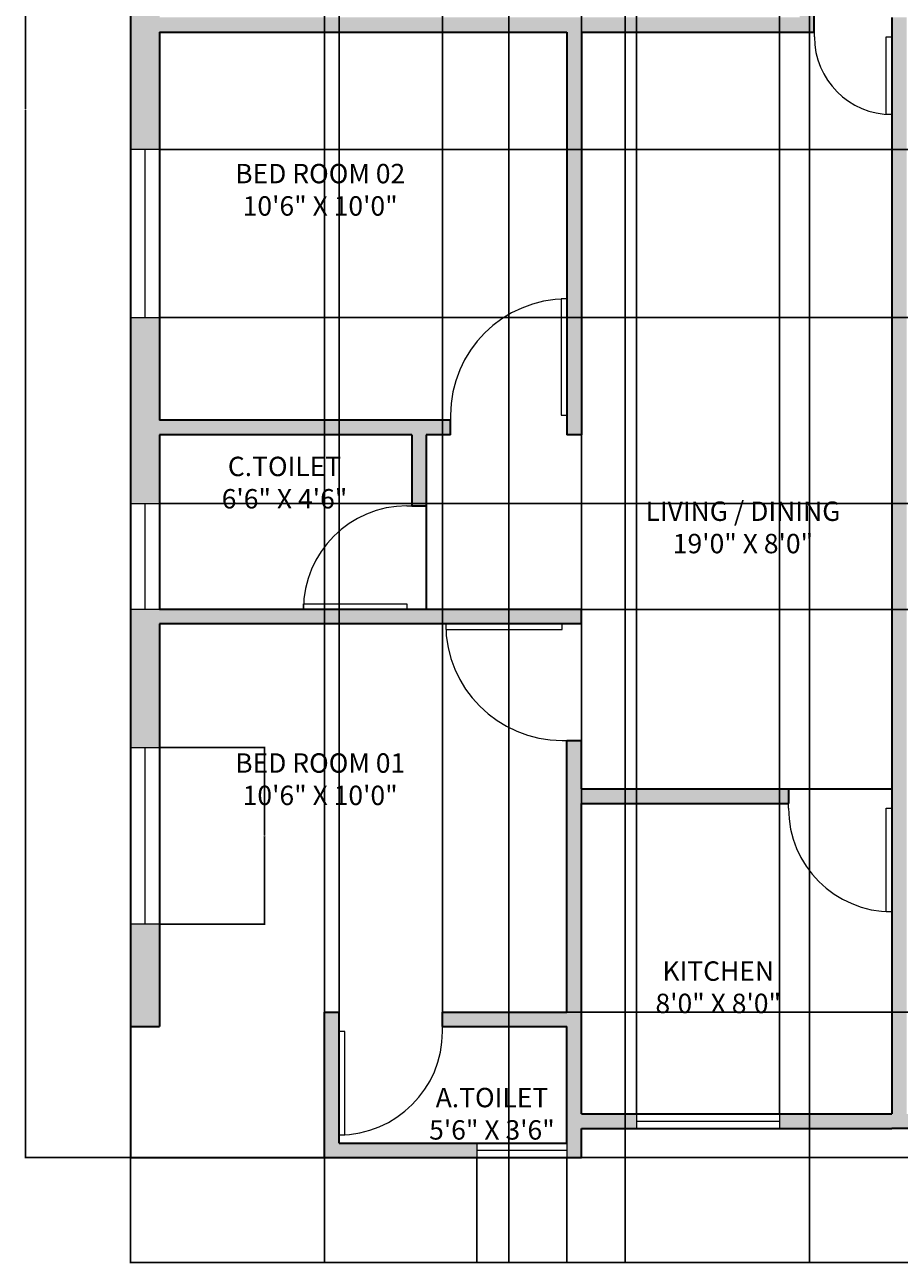
# Model space of a CAD drawing. Units: inches. Extents: x 2510 to 3056, y 673 to 1386.
# Tile 1 of 4: x 2511 to 2781, y 673 to 1056. Entities that reach past the tile are written whole.
import ezdxf

# ---------------------------------------------------------------- set-up
doc = ezdxf.new("R2010")
doc.units = ezdxf.units.IN
for name, color, linetype, lineweight in [('A-ANNO-DIMS', 2, 'Continuous', 18), ('A-AREA-IDEN', 7, 'Continuous', 18), ('A-DOOR', 3, 'Continuous', 18), ('A-GLAZ', 4, 'Continuous', 18), ('A-WALL', 7, 'Continuous', 35), ('A-WALL-PATT', 252, 'Continuous', 13)]:
    doc.layers.add(name, color=color, linetype=linetype, lineweight=lineweight)
doc.styles.get("Standard").update_dxf_attribs({"font": 'arial.ttf'})
doc.dimstyles.get("Standard").update_dxf_attribs({"dimtxt": 0.18, "dimasz": 0.18, "dimexe": 0.18, "dimexo": 0.0625, "dimgap": 0.09, "dimtad": 0, "dimtih": 1, "dimtoh": 1, "dimdec": 4, "dimzin": 0, "dimdsep": 46, "dimtxsty": 'Standard', "dimcen": 0.09, "dimadec": 0, "dimazin": 0, "dimtfac": 1, "dimtdec": 4, "dimtofl": 0, "dimtmove": 0, "dimatfit": 3, "dimfxl": 1, "dimtolj": 1, "dimtzin": 0, "dimarcsym": 0})

# ---------------------------------------------------------------- blocks, each defined once
blk = doc.blocks.new('*U8')
for p, q in [((-24, 0), (-24, 6)), ((0, 0), (0, 6))]:
    blk.add_line(p, q)
blk.add_lwpolyline([(0, 0), (0, -24), (-1.75, -24), (-1.75, 0)], close=True)
blk.add_arc((0, 0), 24, 180, 270)
blk = doc.blocks.new('*U4')
for p, q in [((0, 0), (0, -6)), ((-36, 0), (-36, -6))]:
    blk.add_line(p, q)
blk.add_lwpolyline([(0, 0), (0, 36), (-1.75, 36), (-1.75, 0)], close=True)
blk.add_arc((0, 0), 36, 90, 180)
blk = doc.blocks.new('*U9')
for p, q in [((-32, 0), (-32, 6)), ((0, 0), (0, 6))]:
    blk.add_line(p, q)
blk.add_lwpolyline([(0, 0), (0, -32), (-1.75, -32), (-1.75, 0)], close=True)
blk.add_arc((0, 0), 32, 180, 270)
blk = doc.blocks.new('*U2')
for p, q in [((0, 0), (0, -6)), ((32, 0), (32, -6))]:
    blk.add_line(p, q)
blk.add_lwpolyline([(0, 0), (0, 32), (1.75, 32), (1.75, 0)], close=True)
blk.add_arc((0, 0), 32, 0, 90)
blk = doc.blocks.new('*U5')
for p, q in [((0, 0), (0, 6)), ((32, 0), (32, 6))]:
    blk.add_line(p, q)
blk.add_lwpolyline([(0, 0), (0, -32), (1.75, -32), (1.75, 0)], close=True)
blk.add_arc((0, 0), 32, 270, 0)
blk = doc.blocks.new('*D12')
at = {"layer": 'A-ANNO-DIMS', "color": 0, "lineweight": -2, "transparency": 16777216}
for p, q in [((2543.13, 1353.59), (2510.53, 1353.59)), ((2510.71, 1353.41), (2510.71, 1029.77)), ((2510.71, 705.77), (2510.71, 1029.4)), ((2543.13, 705.59), (2510.53, 705.59))]:
    blk.add_line(p, q, dxfattribs=at)
at = {"layer": 'A-ANNO-DIMS', "color": 0, "transparency": 16777216}
for points in [[(2510.68, 1353.41), (2510.74, 1353.41), (2510.71, 1353.59)], [(2510.68, 705.77), (2510.74, 705.77), (2510.71, 705.59)]]:
    blk.add_solid(points, dxfattribs=at)
at = {"layer": 'Defpoints', "color": 0, "transparency": 16777216}
for p in [(2510.71, 1353.59), (2543.19, 1353.59), (2543.19, 705.59)]:
    blk.add_point(p, dxfattribs=at)
at = {"layer": 'A-ANNO-DIMS', "color": 0, "transparency": 16777216, "insert": (2510.71, 1029.59), "char_height": 0.18, "attachment_point": 5}
blk.add_mtext('\\A1;648', dxfattribs=at)
blk = doc.blocks.new('*D13')
at = {"layer": 'A-ANNO-DIMS', "color": 0, "lineweight": -2, "transparency": 16777216}
for p, q in [((2543.19, 705.52), (2543.19, 672.93)), ((3023.19, 705.52), (3023.19, 672.93)), ((2543.37, 673.11), (2782.9, 673.11)), ((3023.01, 673.11), (2783.48, 673.11))]:
    blk.add_line(p, q, dxfattribs=at)
at = {"layer": 'A-ANNO-DIMS', "color": 0, "transparency": 16777216}
for points in [[(2543.37, 673.14), (2543.37, 673.08), (2543.19, 673.11)], [(3023.01, 673.14), (3023.01, 673.08), (3023.19, 673.11)]]:
    blk.add_solid(points, dxfattribs=at)
at = {"layer": 'Defpoints', "color": 0, "transparency": 16777216}
for p in [(2543.19, 705.59), (3023.19, 705.59), (3023.19, 673.11)]:
    blk.add_point(p, dxfattribs=at)
at = {"layer": 'A-ANNO-DIMS', "color": 0, "transparency": 16777216, "insert": (2783.19, 673.11), "char_height": 0.18, "attachment_point": 5}
blk.add_mtext('\\A1;480', dxfattribs=at)
blk = doc.blocks.new('*D33')
at = {"layer": 'A-ANNO-DIMS', "color": 0, "lineweight": -2, "transparency": 16777216}
for p, q in [((2552.25, 832.37), (2584.85, 832.37)), ((2584.67, 832.19), (2584.67, 805.22)), ((2584.67, 777.9), (2584.67, 804.86)), ((2552.25, 777.72), (2584.85, 777.72))]:
    blk.add_line(p, q, dxfattribs=at)
at = {"layer": 'A-ANNO-DIMS', "color": 0, "transparency": 16777216}
for points in [[(2584.64, 832.19), (2584.7, 832.19), (2584.67, 832.37)], [(2584.64, 777.9), (2584.7, 777.9), (2584.67, 777.72)]]:
    blk.add_solid(points, dxfattribs=at)
at = {"layer": 'Defpoints', "color": 0, "transparency": 16777216}
for p in [(2552.19, 832.37), (2552.19, 777.72), (2584.67, 777.72)]:
    blk.add_point(p, dxfattribs=at)
at = {"layer": 'A-ANNO-DIMS', "color": 0, "transparency": 16777216, "insert": (2584.67, 805.04), "char_height": 0.18, "attachment_point": 5}
blk.add_mtext('\\A1;54.65', dxfattribs=at)
blk = doc.blocks.new('*D34')
at = {"layer": 'A-ANNO-DIMS', "color": 0, "lineweight": -2, "transparency": 16777216}
for p, q in [((2552.25, 907.81), (3055.85, 907.81)), ((3055.67, 907.63), (3055.67, 891.63)), ((3055.67, 875.27), (3055.67, 891.27)), ((2552.25, 875.09), (3055.85, 875.09))]:
    blk.add_line(p, q, dxfattribs=at)
at = {"layer": 'A-ANNO-DIMS', "color": 0, "transparency": 16777216}
for points in [[(3055.64, 907.63), (3055.7, 907.63), (3055.67, 907.81)], [(3055.64, 875.27), (3055.7, 875.27), (3055.67, 875.09)]]:
    blk.add_solid(points, dxfattribs=at)
at = {"layer": 'Defpoints', "color": 0, "transparency": 16777216}
for p in [(2552.19, 907.81), (3055.67, 907.81), (2552.19, 875.09)]:
    blk.add_point(p, dxfattribs=at)
at = {"layer": 'A-ANNO-DIMS', "color": 0, "transparency": 16777216, "insert": (3055.67, 891.45), "char_height": 0.18, "attachment_point": 5}
blk.add_mtext('\\A1;32.72', dxfattribs=at)
blk = doc.blocks.new('*D35')
at = {"layer": 'A-ANNO-DIMS', "color": 0, "lineweight": -2, "transparency": 16777216}
for p, q in [((2552.25, 1017.32), (3055.85, 1017.32)), ((3055.67, 1017.14), (3055.67, 991.52)), ((3055.67, 965.53), (3055.67, 991.15)), ((2552.25, 965.35), (3055.85, 965.35))]:
    blk.add_line(p, q, dxfattribs=at)
at = {"layer": 'A-ANNO-DIMS', "color": 0, "transparency": 16777216}
for points in [[(3055.64, 1017.14), (3055.7, 1017.14), (3055.67, 1017.32)], [(3055.64, 965.53), (3055.7, 965.53), (3055.67, 965.35)]]:
    blk.add_solid(points, dxfattribs=at)
at = {"layer": 'Defpoints', "color": 0, "transparency": 16777216}
for p in [(2552.19, 1017.32), (3055.67, 1017.32), (2552.19, 965.35)]:
    blk.add_point(p, dxfattribs=at)
at = {"layer": 'A-ANNO-DIMS', "color": 0, "transparency": 16777216, "insert": (3055.67, 991.34), "char_height": 0.18, "attachment_point": 5}
blk.add_mtext('\\A1;51.97', dxfattribs=at)
blk = doc.blocks.new('*D40')
at = {"layer": 'A-ANNO-DIMS', "color": 0, "lineweight": -2, "transparency": 16777216}
for p, q in [((2682.69, 719.15), (2682.69, 1386.25)), ((2699.74, 719.15), (2699.74, 1386.25)), ((2682.87, 1386.07), (2690.76, 1386.07)), ((2699.56, 1386.07), (2691.67, 1386.07))]:
    blk.add_line(p, q, dxfattribs=at)
at = {"layer": 'A-ANNO-DIMS', "color": 0, "transparency": 16777216}
for points in [[(2682.87, 1386.1), (2682.87, 1386.04), (2682.69, 1386.07)], [(2699.56, 1386.1), (2699.56, 1386.04), (2699.74, 1386.07)]]:
    blk.add_solid(points, dxfattribs=at)
at = {"layer": 'Defpoints', "color": 0, "transparency": 16777216}
for p in [(2699.74, 1386.07), (2682.69, 719.09), (2699.74, 719.09)]:
    blk.add_point(p, dxfattribs=at)
at = {"layer": 'A-ANNO-DIMS', "color": 0, "transparency": 16777216, "insert": (2691.22, 1386.07), "char_height": 0.18, "attachment_point": 5}
blk.add_mtext('\\A1;17.045', dxfattribs=at)
blk = doc.blocks.new('*D41')
at = {"layer": 'A-ANNO-DIMS', "color": 0, "lineweight": -2, "transparency": 16777216}
for p, q in [((2699.74, 719.15), (2699.74, 1386.25)), ((2743.88, 719.15), (2743.88, 1386.25)), ((2699.92, 1386.07), (2721.41, 1386.07)), ((2743.7, 1386.07), (2722.21, 1386.07))]:
    blk.add_line(p, q, dxfattribs=at)
at = {"layer": 'A-ANNO-DIMS', "color": 0, "transparency": 16777216}
for points in [[(2699.92, 1386.1), (2699.92, 1386.04), (2699.74, 1386.07)], [(2743.7, 1386.1), (2743.7, 1386.04), (2743.88, 1386.07)]]:
    blk.add_solid(points, dxfattribs=at)
at = {"layer": 'Defpoints', "color": 0, "transparency": 16777216}
for p in [(2743.88, 1386.07), (2699.74, 719.09), (2743.88, 719.09)]:
    blk.add_point(p, dxfattribs=at)
at = {"layer": 'A-ANNO-DIMS', "color": 0, "transparency": 16777216, "insert": (2721.81, 1386.07), "char_height": 0.18, "attachment_point": 5}
blk.add_mtext('\\A1;44.14', dxfattribs=at)
blk = doc.blocks.new('*D45')
at = {"layer": 'A-ANNO-DIMS', "color": 0, "lineweight": -2, "transparency": 16777216}
for p, q in [((2660.19, 1208.02), (2660.19, 672.93)), ((2696.19, 1208.02), (2696.19, 672.93)), ((2660.37, 673.11), (2677.97, 673.11)), ((2696.01, 673.11), (2678.41, 673.11))]:
    blk.add_line(p, q, dxfattribs=at)
at = {"layer": 'A-ANNO-DIMS', "color": 0, "transparency": 16777216}
for points in [[(2660.37, 673.14), (2660.37, 673.08), (2660.19, 673.11)], [(2696.01, 673.14), (2696.01, 673.08), (2696.19, 673.11)]]:
    blk.add_solid(points, dxfattribs=at)
at = {"layer": 'Defpoints', "color": 0, "transparency": 16777216}
for p in [(2660.19, 1208.09), (2696.19, 1208.09), (2696.19, 673.11)]:
    blk.add_point(p, dxfattribs=at)
at = {"layer": 'A-ANNO-DIMS', "color": 0, "transparency": 16777216, "insert": (2678.19, 673.11), "char_height": 0.18, "attachment_point": 5}
blk.add_mtext('\\A1;36', dxfattribs=at)
blk = doc.blocks.new('*D46')
at = {"layer": 'A-ANNO-DIMS', "color": 0, "lineweight": -2, "transparency": 16777216}
for p, q in [((2753.19, 1256.02), (2753.19, 672.93)), ((2785.19, 1256.02), (2785.19, 672.93)), ((2753.37, 673.11), (2768.97, 673.11)), ((2785.01, 673.11), (2769.41, 673.11))]:
    blk.add_line(p, q, dxfattribs=at)
at = {"layer": 'A-ANNO-DIMS', "color": 0, "transparency": 16777216}
for points in [[(2753.37, 673.14), (2753.37, 673.08), (2753.19, 673.11)], [(2785.01, 673.14), (2785.01, 673.08), (2785.19, 673.11)]]:
    blk.add_solid(points, dxfattribs=at)
at = {"layer": 'Defpoints', "color": 0, "transparency": 16777216}
for p in [(2753.19, 1256.09), (2785.19, 1256.09), (2785.19, 673.11)]:
    blk.add_point(p, dxfattribs=at)
at = {"layer": 'A-ANNO-DIMS', "color": 0, "transparency": 16777216, "insert": (2769.19, 673.11), "char_height": 0.18, "attachment_point": 5}
blk.add_mtext('\\A1;32', dxfattribs=at)
blk = doc.blocks.new('*D50')
at = {"layer": 'A-ANNO-DIMS', "color": 0, "lineweight": -2, "transparency": 16777216}
for p, q in [((2607.69, 750.65), (2607.69, 1386.25)), ((2639.69, 750.65), (2639.69, 1386.25)), ((2607.87, 1386.07), (2623.47, 1386.07)), ((2639.51, 1386.07), (2623.91, 1386.07))]:
    blk.add_line(p, q, dxfattribs=at)
at = {"layer": 'A-ANNO-DIMS', "color": 0, "transparency": 16777216}
for points in [[(2607.87, 1386.1), (2607.87, 1386.04), (2607.69, 1386.07)], [(2639.51, 1386.1), (2639.51, 1386.04), (2639.69, 1386.07)]]:
    blk.add_solid(points, dxfattribs=at)
at = {"layer": 'Defpoints', "color": 0, "transparency": 16777216}
for p in [(2639.69, 1386.07), (2607.69, 750.59), (2639.69, 750.59)]:
    blk.add_point(p, dxfattribs=at)
at = {"layer": 'A-ANNO-DIMS', "color": 0, "transparency": 16777216, "insert": (2623.69, 1386.07), "char_height": 0.18, "attachment_point": 5}
blk.add_mtext('\\A1;32', dxfattribs=at)
blk = doc.blocks.new('*D51')
at = {"layer": 'A-ANNO-DIMS', "color": 0, "lineweight": -2, "transparency": 16777216}
for p, q in [((2650.28, 705.52), (2650.28, 672.93)), ((2678.19, 705.52), (2678.19, 672.93)), ((2650.46, 673.11), (2663.77, 673.11)), ((2678.01, 673.11), (2664.7, 673.11))]:
    blk.add_line(p, q, dxfattribs=at)
at = {"layer": 'A-ANNO-DIMS', "color": 0, "transparency": 16777216}
for points in [[(2650.46, 673.14), (2650.46, 673.08), (2650.28, 673.11)], [(2678.01, 673.14), (2678.01, 673.08), (2678.19, 673.11)]]:
    blk.add_solid(points, dxfattribs=at)
at = {"layer": 'Defpoints', "color": 0, "transparency": 16777216}
for p in [(2650.28, 705.59), (2678.19, 705.59), (2678.19, 673.11)]:
    blk.add_point(p, dxfattribs=at)
at = {"layer": 'A-ANNO-DIMS', "color": 0, "transparency": 16777216, "insert": (2664.23, 673.11), "char_height": 0.18, "attachment_point": 5}
blk.add_mtext('\\A1;27.916', dxfattribs=at)
blk = doc.blocks.new('*D52')
at = {"layer": 'A-ANNO-DIMS', "color": 0, "lineweight": -2, "transparency": 16777216}
for p, q in [((2603.19, 705.52), (2603.19, 672.93)), ((2650.28, 705.52), (2650.28, 672.93)), ((2603.37, 673.11), (2626.34, 673.11)), ((2650.1, 673.11), (2627.13, 673.11))]:
    blk.add_line(p, q, dxfattribs=at)
at = {"layer": 'A-ANNO-DIMS', "color": 0, "transparency": 16777216}
for points in [[(2603.37, 673.14), (2603.37, 673.08), (2603.19, 673.11)], [(2650.1, 673.14), (2650.1, 673.08), (2650.28, 673.11)]]:
    blk.add_solid(points, dxfattribs=at)
at = {"layer": 'Defpoints', "color": 0, "transparency": 16777216}
for p in [(2603.19, 705.59), (2650.28, 705.59), (2650.28, 673.11)]:
    blk.add_point(p, dxfattribs=at)
at = {"layer": 'A-ANNO-DIMS', "color": 0, "transparency": 16777216, "insert": (2626.73, 673.11), "char_height": 0.18, "attachment_point": 5}
blk.add_mtext('\\A1;47.08', dxfattribs=at)
blk = doc.blocks.new('*D53')
at = {"layer": 'A-ANNO-DIMS', "color": 0, "lineweight": -2, "transparency": 16777216}
for p, q in [((2682.75, 714.59), (3055.85, 714.59)), ((3055.67, 714.41), (3055.67, 710.27)), ((3055.67, 705.77), (3055.67, 709.9)), ((2682.75, 705.59), (3055.85, 705.59))]:
    blk.add_line(p, q, dxfattribs=at)
at = {"layer": 'A-ANNO-DIMS', "color": 0, "transparency": 16777216}
for points in [[(3055.64, 714.41), (3055.7, 714.41), (3055.67, 714.59)], [(3055.64, 705.77), (3055.7, 705.77), (3055.67, 705.59)]]:
    blk.add_solid(points, dxfattribs=at)
at = {"layer": 'Defpoints', "color": 0, "transparency": 16777216}
for p in [(2682.69, 714.59), (3055.67, 714.59), (2682.69, 705.59)]:
    blk.add_point(p, dxfattribs=at)
at = {"layer": 'A-ANNO-DIMS', "color": 0, "transparency": 16777216, "insert": (3055.67, 710.09), "char_height": 0.18, "attachment_point": 5}
blk.add_mtext('\\A1;9', dxfattribs=at)
blk = doc.blocks.new('*D54')
at = {"layer": 'A-ANNO-DIMS', "color": 0, "lineweight": -2, "transparency": 16777216}
for p, q in [((2678.25, 750.59), (3055.85, 750.59)), ((3055.67, 750.41), (3055.67, 732.77)), ((3055.67, 714.77), (3055.67, 732.4)), ((2682.75, 714.59), (3055.85, 714.59))]:
    blk.add_line(p, q, dxfattribs=at)
at = {"layer": 'A-ANNO-DIMS', "color": 0, "transparency": 16777216}
for points in [[(3055.64, 750.41), (3055.7, 750.41), (3055.67, 750.59)], [(3055.64, 714.77), (3055.7, 714.77), (3055.67, 714.59)]]:
    blk.add_solid(points, dxfattribs=at)
at = {"layer": 'Defpoints', "color": 0, "transparency": 16777216}
for p in [(2678.19, 750.59), (3055.67, 750.59), (2682.69, 714.59)]:
    blk.add_point(p, dxfattribs=at)
at = {"layer": 'A-ANNO-DIMS', "color": 0, "transparency": 16777216, "insert": (3055.67, 732.59), "char_height": 0.18, "attachment_point": 5}
blk.add_mtext('\\A1;36', dxfattribs=at)
blk = doc.blocks.new('*D57')
at = {"layer": 'A-ANNO-DIMS', "color": 0, "lineweight": -2, "transparency": 16777216}
for p, q in [((2543.19, 705.65), (2543.19, 1386.25)), ((2603.19, 705.65), (2603.19, 1386.25)), ((2543.37, 1386.07), (2572.97, 1386.07)), ((2603.01, 1386.07), (2573.41, 1386.07))]:
    blk.add_line(p, q, dxfattribs=at)
at = {"layer": 'A-ANNO-DIMS', "color": 0, "transparency": 16777216}
for points in [[(2543.37, 1386.1), (2543.37, 1386.04), (2543.19, 1386.07)], [(2603.01, 1386.1), (2603.01, 1386.04), (2603.19, 1386.07)]]:
    blk.add_solid(points, dxfattribs=at)
at = {"layer": 'Defpoints', "color": 0, "transparency": 16777216}
for p in [(2603.19, 1386.07), (2543.19, 705.59), (2603.19, 705.59)]:
    blk.add_point(p, dxfattribs=at)
at = {"layer": 'A-ANNO-DIMS', "color": 0, "transparency": 16777216, "insert": (2573.19, 1386.07), "char_height": 0.18, "attachment_point": 5}
blk.add_mtext('\\A1;60', dxfattribs=at)

msp = doc.modelspace()

# ---------------------------------------------------------------- hatches: boundary and pattern name
at = {"layer": 'A-WALL-PATT'}
h = msp.add_hatch(color=256, dxfattribs=at)
h.dxf.hatch_style = 1
h.paths.add_polyline_path([(2580.5162, 1353.5862), (2543.1924, 1353.5862), (2543.1924, 1311.5591), (2552.1924, 1311.5591), (2552.1924, 1344.5862), (2580.5162, 1344.5862)])
h.paths.add_polyline_path([(2720.7125, 1353.5862), (2648.0497, 1353.5862), (2648.0497, 1344.5862), (2696.1924, 1344.5862), (2696.1924, 1208.0862), (2700.6924, 1208.0862), (2700.6924, 1256.0862), (2716.6924, 1256.0862), (2716.6924, 1260.5862), (2700.6924, 1260.5862), (2700.6924, 1344.5862), (2720.7125, 1344.5862)])
h.paths.add_polyline_path([(2762.4727, 1353.5862), (2748.6924, 1353.5862), (2748.6924, 1344.5862), (2748.6924, 1256.0862), (2753.1924, 1256.0862), (2753.1924, 1262.0862), (2753.1924, 1294.0862), (2753.1924, 1344.5862), (2762.4727, 1344.5862)])
h.paths.add_polyline_path([(2863.5016, 1353.5862), (2808.6621, 1353.5862), (2808.6621, 1344.5862), (2825.1924, 1344.5862), (2825.1924, 1260.5862), (2785.1924, 1260.5862), (2785.1924, 1256.0862), (2825.1924, 1256.0862), (2825.1924, 1248.5862), (2829.6924, 1248.5862), (2829.6924, 1344.5862), (2863.5016, 1344.5862)])
h.paths.add_polyline_path([(2966.1924, 1353.5862), (2915.7284, 1353.5862), (2915.7284, 1344.5862), (2961.6924, 1344.5862), (2961.6924, 1212.5862), (2897.6924, 1212.5862), (2897.6924, 1208.0862), (2961.6924, 1208.0862), (2961.6924, 1193.4346), (2966.1924, 1193.4346), (2966.1924, 1208.0862)])
h.paths.add_polyline_path([(2660.1924, 1212.5862), (2552.1924, 1212.5862), (2552.1924, 1254.8401), (2543.1924, 1254.8401), (2543.1924, 1168.7504), (2552.1924, 1168.7504), (2552.1924, 1208.0862), (2660.1924, 1208.0862)])
h.paths.add_polyline_path([(3023.1924, 1160.0862), (2966.1924, 1160.0862), (2966.1924, 1165.033), (2961.6924, 1165.033), (2961.6924, 1160.0862), (2865.6924, 1160.0862), (2865.6924, 1212.5862), (2825.1924, 1212.5862), (2825.1924, 1208.0862), (2861.1924, 1208.0862), (2861.1924, 1160.0862), (2750.1527, 1160.0862), (2750.1527, 1155.5862), (2754.6527, 1155.5862), (2966.1924, 1155.5862), (3014.1924, 1155.5862), (3014.1924, 1136.4806), (3023.1924, 1136.4806)])
h.paths.add_polyline_path([(3023.1924, 1090.8839), (3014.1924, 1090.8839), (3014.1924, 1058.0862), (2807.1924, 1058.0862), (2807.1924, 1053.5862), (2879.1924, 1053.5862), (2879.1924, 929.0862), (2883.6924, 929.0862), (2883.6924, 935.0862), (2883.6924, 971.0862), (2883.6924, 1053.5862), (3014.1924, 1053.5862), (3014.1924, 1028.0329), (3023.1924, 1028.0329)])
h.paths.add_polyline_path([(3023.1924, 970.6943), (3014.1924, 970.6943), (3014.1924, 933.5862), (2919.6924, 933.5862), (2919.6924, 929.0862), (2927.1924, 929.0862), (2927.1924, 907.0862), (2931.6924, 907.0862), (2931.6924, 929.0862), (3014.1924, 929.0862), (3014.1924, 918.5377), (3023.1924, 918.5377)])
h.paths.add_polyline_path([(3023.1924, 886.219), (3014.1924, 886.219), (3014.1924, 875.0862), (2927.1924, 875.0862), (2879.1924, 875.0862), (2879.1924, 870.5862), (2885.1924, 870.5862), (2921.1924, 870.5862), (3014.1924, 870.5862), (3014.1924, 835.4806), (3023.1924, 835.4806)])
h.paths.add_polyline_path([(3023.1924, 775.6299), (3014.1924, 775.6299), (3014.1924, 746.0862), (3023.1924, 746.0862)])
h.paths.add_polyline_path([(2958.6924, 750.5862), (2954.1924, 750.5862), (2954.1924, 744.5862), (2954.1924, 716.5862), (2954.1924, 710.0862), (2910.6841, 710.0862), (2910.6841, 705.5862), (2958.6924, 705.5862)])
h.paths.add_polyline_path([(2926.1924, 750.5862), (2883.6924, 750.5862), (2883.6924, 834.5862), (2879.1924, 834.5862), (2879.1924, 819.5862), (2815.1924, 819.5862), (2815.1924, 815.0862), (2879.1924, 815.0862), (2879.1924, 746.0862), (2879.1924, 719.0862), (2862.8388, 719.0862), (2862.8388, 714.5862), (2879.1924, 714.5862), (2879.1924, 705.5862), (2883.6924, 705.5862), (2883.6924, 710.0862), (2883.6924, 746.0862), (2926.1924, 746.1758)])
h.paths.add_polyline_path([(2682.6924, 815.0862), (2746.6924, 815.0862), (2746.6924, 819.5862), (2682.6924, 819.5862), (2682.6924, 834.5862), (2678.1924, 834.5862), (2678.1924, 750.5862), (2639.6924, 750.5862), (2639.6924, 746.0862), (2678.1924, 746.0862), (2678.1924, 710.0862), (2678.1924, 705.5862), (2682.6924, 705.5862), (2682.6924, 714.5862), (2699.7376, 714.5862), (2699.7376, 719.0862), (2682.6924, 719.0862), (2682.6924, 746.0862)])
h.paths.add_polyline_path([(2650.2761, 710.0862), (2607.6924, 710.0862), (2607.6924, 750.5862), (2603.1924, 750.5862), (2603.1924, 705.5862), (2607.6924, 705.5862), (2650.2761, 705.5862)])
h.paths.add_polyline_path([(2552.1924, 777.7158), (2543.1924, 777.7158), (2543.1924, 746.0862), (2552.1924, 746.0862)])
h.paths.add_polyline_path([(2828.3093, 719.0862), (2783.1924, 719.0862), (2783.1924, 815.0862), (2783.1924, 1058.0862), (2778.6924, 1058.0862), (2778.6924, 815.0862), (2778.6924, 719.0862), (2743.8813, 719.0862), (2743.8813, 714.5862), (2778.6924, 714.5862), (2828.3093, 714.5862)])
h.paths.add_polyline_path([(2642.1924, 933.5862), (2552.1924, 933.5862), (2552.1924, 965.3494), (2543.1924, 965.3494), (2543.1924, 907.809), (2552.1924, 907.809), (2552.1924, 929.0862), (2630.1924, 929.0862), (2630.1924, 907.0862), (2634.6924, 907.0862), (2634.6924, 929.0862), (2642.1924, 929.0862)])
h.paths.add_polyline_path([(2682.6924, 875.0862), (2552.1924, 875.0862), (2543.1924, 875.0862), (2543.1924, 832.3664), (2552.1924, 832.3664), (2552.1924, 870.5862), (2634.6924, 870.5862), (2682.6924, 870.5862)])
h.paths.add_polyline_path([(2754.6527, 1119.5862), (2750.1527, 1119.5862), (2750.1527, 1058.0862), (2552.1924, 1058.0862), (2552.1924, 1104.0128), (2543.1924, 1104.0128), (2543.1924, 1017.3235), (2552.1924, 1017.3235), (2552.1924, 1053.5862), (2678.1924, 1053.5862), (2678.1924, 929.0862), (2682.6924, 929.0862), (2682.6924, 1053.5862), (2754.6527, 1053.5862)])

# ---------------------------------------------------------------- linework, layer by layer
at = {"layer": 'A-GLAZ'}
for p, q in [((2543.1924, 1017.3235), (2552.1924, 1017.3235)), ((2547.6924, 965.3494), (2547.6924, 1017.3235)), ((2543.1924, 965.3494), (2552.1924, 965.3494)), ((2543.1924, 907.809), (2552.1924, 907.809)), ((2547.6924, 875.0862), (2547.6924, 907.809)), ((2552.1924, 875.0862), (2543.1924, 875.0862)), ((2543.1924, 832.3664), (2552.1924, 832.3664)), ((2547.6924, 777.7158), (2547.6924, 832.3664)), ((2552.1924, 777.7158), (2543.1924, 777.7158)), ((2699.7376, 719.0862), (2699.7376, 714.5862)), ((2699.7376, 716.8362), (2743.8813, 716.8362)), ((2743.8813, 719.0862), (2743.8813, 714.5862)), ((2650.2761, 710.0862), (2650.2761, 705.5862)), ((2678.1924, 710.0862), (2678.1924, 705.5862)), ((2650.2761, 707.8362), (2678.1924, 707.8362))]:
    msp.add_line(p, q, dxfattribs=at)
at = {"layer": 'A-WALL'}
for p, q in [((2543.1924, 1353.5862), (2543.1924, 705.5862)), ((2754.6527, 1053.5862), (2754.6527, 1119.5862)), ((2778.6924, 1058.0862), (2778.6924, 815.0862)), ((2552.1924, 1053.5862), (2678.1924, 1053.5862)), ((2552.1924, 1053.5862), (2552.1924, 933.5862)), ((2678.1924, 1053.5862), (2678.1924, 929.0862)), ((2682.6924, 1053.5862), (2682.6924, 929.0862)), ((2682.6924, 1053.5862), (2754.6527, 1053.5862)), ((2642.1924, 933.5862), (2552.1924, 933.5862)), ((2642.1924, 929.0862), (2642.1924, 933.5862)), ((2630.1924, 929.0862), (2552.1924, 929.0862)), ((2552.1924, 929.0862), (2552.1924, 875.0862)), ((2630.1924, 929.0862), (2630.1924, 907.0862)), ((2634.6924, 929.0862), (2634.6924, 875.0862)), ((2642.1924, 929.0862), (2634.6924, 929.0862)), ((2682.6924, 929.0862), (2678.1924, 929.0862)), ((2630.1924, 907.0862), (2634.6924, 907.0862)), ((2682.6924, 875.0862), (2552.1924, 875.0862)), ((2682.6924, 870.5862), (2682.6924, 875.0862)), ((2634.6924, 870.5862), (2552.1924, 870.5862)), ((2552.1924, 870.5862), (2552.1924, 746.0862)), ((2682.6924, 870.5862), (2634.6924, 870.5862)), ((2678.1924, 750.5862), (2678.1924, 834.5862)), ((2678.1924, 834.5862), (2682.6924, 834.5862)), ((2682.6924, 819.5862), (2682.6924, 834.5862)), ((2682.6924, 819.5862), (2778.6924, 819.5862)), ((2746.6924, 819.5862), (2746.6924, 815.0862)), ((2682.6924, 746.0862), (2682.6924, 815.0862)), ((2682.6924, 815.0862), (2746.6924, 815.0862)), ((2778.6924, 815.0862), (2778.6924, 719.0862)), ((2603.1924, 750.5862), (2607.6924, 750.5862)), ((2603.1924, 705.5862), (2603.1924, 750.5862)), ((2607.6924, 710.0862), (2607.6924, 750.5862)), ((2639.6924, 746.0862), (2639.6924, 750.5862)), ((2639.6924, 750.5862), (2678.1924, 750.5862)), ((2543.1924, 746.0862), (2552.1924, 746.0862)), ((2639.6924, 746.0862), (2678.1924, 746.0862)), ((2678.1924, 710.0862), (2678.1924, 746.0862)), ((2682.6924, 719.0862), (2682.6924, 746.0862)), ((2682.6924, 719.0862), (2778.6924, 719.0862)), ((2682.6924, 705.5862), (2682.6924, 714.5862)), ((2682.6924, 714.5862), (2778.6924, 714.5862)), ((2879.1924, 714.5862), (2778.6924, 714.5862)), ((2607.6924, 710.0862), (2678.1924, 710.0862)), ((2543.1924, 705.5862), (2603.1924, 705.5862)), ((2603.1924, 705.5862), (2607.6924, 705.5862)), ((2607.6924, 705.5862), (2678.1924, 705.5862)), ((2678.1924, 705.5862), (2682.6924, 705.5862))]:
    msp.add_line(p, q, dxfattribs=at)

# ---------------------------------------------------------------- block references
at = {"layer": 'A-DOOR'}
for name, p in [('*U8', (2778.6924, 1052.0862)), ('*U4', (2678.1924, 935.0862)), ('*U9', (2778.6924, 813.5862)), ('*U5', (2607.6924, 744.5862))]:
    msp.add_blockref(name, p, dxfattribs=at)
at = {"layer": 'A-DOOR', "rotation": 90}
for name, p in [('*U2', (2628.6924, 875.0862)), ('*U4', (2676.6924, 870.5862))]:
    msp.add_blockref(name, p, dxfattribs=at)

# ---------------------------------------------------------------- texts
at = {"layer": 'A-AREA-IDEN', "char_height": 6, "attachment_point": 1}
for s, width, insert in [('\\pxqc;BED ROOM 02\\P10\'6" X 10\'0"', 59.569763, (2572.0833, 1012.8204)), ('\\pxqc;C.TOILET\\P6\'6" X 4\'6"', 59.569763, (2561.0461, 922.2835)), ('\\pxqc;LIVING / DINING\\P19\'0" X 8\'0"', 75.716205, (2694.7584, 908.4349)), ('\\pxqc;BED ROOM 01\\P10\'6" X 10\'0"', 59.569763, (2572.0833, 830.5806)), ('\\pxqc;KITCHEN\\P\\pt7;8\'0" X 8\'0"', 59.569763, (2695.1869, 766.2581)), ('\\pxqc;A.TOILET\\P5\'6" X 3\'6"', 40.931341, (2634.522, 727.1456))]:
    msp.add_mtext_dynamic_manual_height_columns(s, width=width, gutter_width=12.5, heights=[0], dxfattribs=dict(at, insert=insert))

# ---------------------------------------------------------------- dimensions: what is measured, and where the dimension line sits
at = {"layer": 'A-ANNO-DIMS'}
for base, p1, p2, override, picture, middle in [((2603.1924, 1386.0667), (2543.1924, 705.5862), (2603.1924, 705.5862), {"dimdec": 0, "dimlfac": 1, "dimrnd": 0, "dimzin": 0, "dimdsep": 46, "dimlunit": 2}, '*D57', (2573.1924, 1386.0667)), ((2639.6924, 1386.0667), (2607.6924, 750.5862), (2639.6924, 750.5862), {"dimdec": 0, "dimlfac": 1, "dimrnd": 0, "dimzin": 0, "dimdsep": 46, "dimlunit": 2}, '*D50', (2623.6924, 1386.0667)), ((2699.7376, 1386.0667), (2682.6924, 719.0862), (2699.7376, 719.0862), {"dimdec": 3, "dimlfac": 1, "dimrnd": 0, "dimzin": 0, "dimdsep": 46, "dimlunit": 2}, '*D40', (2691.215, 1386.0667)), ((2743.8813, 1386.0667), (2699.7376, 719.0862), (2743.8813, 719.0862), {"dimdec": 2, "dimlfac": 1, "dimrnd": 0, "dimzin": 0, "dimdsep": 46, "dimlunit": 2}, '*D41', (2721.8095, 1386.0667)), ((2785.1924, 673.1057), (2753.1924, 1256.0862), (2785.1924, 1256.0862), {"dimdec": 0, "dimlfac": 1, "dimrnd": 0, "dimzin": 0, "dimdsep": 46, "dimlunit": 2}, '*D46', (2769.1924, 673.1057)), ((2696.1924, 673.1057), (2660.1924, 1208.0862), (2696.1924, 1208.0862), {"dimdec": 0, "dimlfac": 1, "dimrnd": 0, "dimzin": 0, "dimdsep": 46, "dimlunit": 2}, '*D45', (2678.1924, 673.1057)), ((3023.1924, 673.1057), (2543.1924, 705.5862), (3023.1924, 705.5862), {"dimdec": 0, "dimlfac": 1, "dimrnd": 0, "dimzin": 0, "dimdsep": 46, "dimlunit": 2}, '*D13', (2783.1924, 673.1057)), ((2650.2761, 673.1057), (2603.1924, 705.5862), (2650.2761, 705.5862), {"dimdec": 2, "dimlfac": 1, "dimrnd": 0, "dimzin": 0, "dimdsep": 46, "dimlunit": 2}, '*D52', (2626.7343, 673.1057)), ((2678.1924, 673.1057), (2650.2761, 705.5862), (2678.1924, 705.5862), {"dimdec": 3, "dimlfac": 1, "dimrnd": 0, "dimzin": 0, "dimdsep": 46, "dimlunit": 2}, '*D51', (2664.2343, 673.1057))]:
    dim = msp.add_linear_dim(base=base, p1=p1, p2=p2, dimstyle='Standard', override=override, dxfattribs=at)
    dim.commit()
    dim.dimension.update_dxf_attribs({"geometry": picture, "text_midpoint": middle})
for base, p1, p2, angle, override, picture, middle in [((2510.7119, 1353.5862), (2543.1924, 705.5862), (2543.1924, 1353.5862), 90, {"dimdec": 0, "dimlfac": 1, "dimrnd": 0, "dimzin": 0, "dimdsep": 46, "dimlunit": 2}, '*D12', (2510.7119, 1029.5862)), ((3055.6729, 1017.3235), (2552.1924, 965.3494), (2552.1924, 1017.3235), 90, {"dimdec": 2, "dimlfac": 1, "dimrnd": 0, "dimzin": 0, "dimdsep": 46, "dimlunit": 2}, '*D35', (3055.6729, 991.3364)), ((3055.6729, 907.809), (2552.1924, 875.0862), (2552.1924, 907.809), 90, {"dimdec": 2, "dimlfac": 1, "dimrnd": 0, "dimzin": 0, "dimdsep": 46, "dimlunit": 2}, '*D34', (3055.6729, 891.4476)), ((2584.6729, 777.7158), (2552.1924, 832.3664), (2552.1924, 777.7158), 270, {"dimdec": 2, "dimlfac": 1, "dimrnd": 0, "dimzin": 0, "dimdsep": 46, "dimlunit": 2}, '*D33', (2584.6729, 805.0411)), ((3055.6729, 750.5862), (2682.6924, 714.5862), (2678.1924, 750.5862), 90, {"dimdec": 0, "dimlfac": 1, "dimrnd": 0, "dimzin": 0, "dimdsep": 46, "dimlunit": 2}, '*D54', (3055.6729, 732.5862)), ((3055.6729, 714.5862), (2682.6924, 705.5862), (2682.6924, 714.5862), 90, {"dimdec": 0, "dimlfac": 1, "dimrnd": 0, "dimzin": 0, "dimdsep": 46, "dimlunit": 2}, '*D53', (3055.6729, 710.0862))]:
    dim = msp.add_linear_dim(base=base, p1=p1, p2=p2, angle=angle, dimstyle='Standard', override=override, dxfattribs=at)
    dim.commit()
    dim.dimension.update_dxf_attribs({"geometry": picture, "text_midpoint": middle})

doc.saveas('drawing.dxf')
